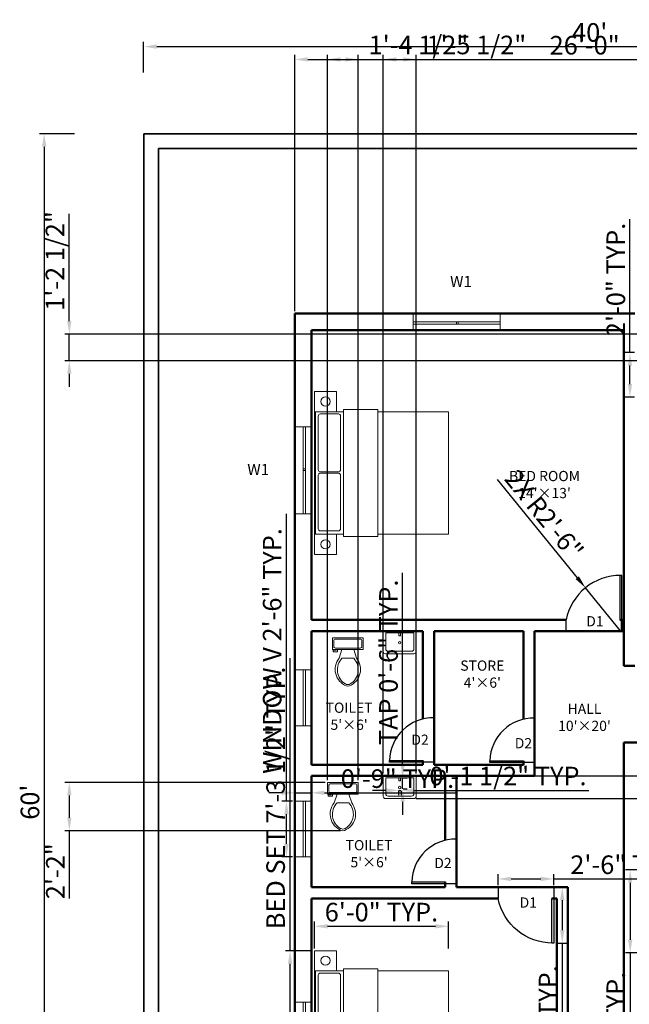
# Model space of a CAD drawing. Units: inches. Extents: x 452 to 1041, y 578 to 1412.
# Tile 2 of 3: x 452 to 780, y 881 to 1412. Entities that reach past the tile are written whole.
import ezdxf

# ---------------------------------------------------------------- set-up
doc = ezdxf.new("R2010")
doc.units = ezdxf.units.IN
doc.linetypes.add('ACAD_ISO03W100', pattern=[30, 12, -18])
doc.layers.get('Defpoints').update_dxf_attribs({"linetype": 'ACAD_ISO03W100'})
for name, color, linetype, lineweight in [('A-ANNO-DIMS', 2, 'Continuous', 18), ('A-ANNO-TEXT', 7, 'Continuous', 18), ('A-AREA-IDEN', 7, 'Continuous', 25), ('A-DOOR', 3, 'Continuous', 25), ('A-FLOR-FIXT', 9, 'Continuous', 18), ('A-FURN', 8, 'Continuous', 18), ('A-GLAZ', 160, 'Continuous', 20), ('A-WALL', 7, 'Continuous', 50), ('C-PROP', 7, 'Continuous', 35)]:
    doc.layers.add(name, color=color, linetype=linetype, lineweight=lineweight)
doc.styles.get("Standard").update_dxf_attribs({"font": 'times.ttf'})
doc.dimstyles.new('ISO-25', dxfattribs={"dimscale": 2, "dimtxt": 5, "dimasz": 3.5, "dimexe": 1.25, "dimexo": 0.625, "dimtad": 1, "dimdsep": 46, "dimlunit": 3, "dimtxsty": 'Standard', "dimcen": 2.5, "dimadec": 0, "dimazin": 0, "dimtfac": 1, "dimtmove": 0, "dimatfit": 3, "dimfxl": 1, "dimarcsym": 0})

# ---------------------------------------------------------------- blocks, each defined once
blk = doc.blocks.new('*U2')
for p, q in [((9.5, -6), (9.5, -2)), ((-10, -8.5), (-8, -8.5)), ((-10, -9.5), (-10, -8.5)), ((-7, -9.5), (-10, -9.5)), ((-8, -8.5), (-8, -8)), ((-7, -8), (-7, -9.5)), ((-4, -8), (-6, -14)), ((4, -8), (6, -14)), ((4, -14), (-4, -14))]:
    blk.add_line(p, q)
blk.add_lwpolyline([(10.5, -8), (10.5, 0), (-10.5, 0), (-10.5, -8)], close=True)
for points in [[(-9.5, -2), (-9.5, -6)], [(8.5, -1), (-8.5, -1)], [(-8.5, -7), (8.5, -7)]]:
    blk.add_lwpolyline(points)
for centre, radius, start, end in [((-8.62, -1.88), 0.884, 81.8699, 188.1301), ((-8.62, -6.12), 0.884, 171.8699, 278.1301), ((8.62, -1.88), 0.884, 351.8699, 98.1301), ((8.62, -6.12), 0.884, 261.8699, 8.1301), ((3.52, -21.58), 12.17, 141.46911, 247.97143), ((4.2, -21.82), 11.33, 136.36773, 238.94682), ((-3.52, -21.58), 12.17, 292.02843, 38.53071), ((-4.2, -21.82), 11.33, 301.05301, 43.63209), ((0, -27.88), 4, 245.73182, 294.26817), ((0, -29), 4, 254.86053, 285.13947)]:
    blk.add_arc(centre, radius, start, end)
blk = doc.blocks.new('D1')
for p, q in [((734.6, 1191.77), (733.6, 1191.77)), ((733.6, 1191.77), (733.6, 1167.77)), ((734.6, 1161.77), (734.6, 1191.77)), ((704.6, 1161.77), (704.6, 1167.77))]:
    blk.add_line(p, q)
blk.add_arc((733.85, 1161.94), 29.82, 89.5197, 168.7411)
blk = doc.blocks.new('W')
for p, q in [((913.24, 916.29), (913.24, 963.09)), ((913.24, 963.09), (922.24, 963.09)), ((917.74, 963.09), (917.74, 916.29)), ((918.94, 963.09), (918.94, 916.29)), ((922.24, 963.09), (922.24, 916.29)), ((917.74, 940.48), (918.94, 940.48)), ((917.74, 939.69), (918.94, 939.69)), ((922.24, 916.29), (913.24, 916.29))]:
    blk.add_line(p, q)
blk = doc.blocks.new('V')
for p, q in [((599.59, 961.66), (599.59, 991.66)), ((599.59, 991.66), (608.59, 991.66)), ((604.09, 961.66), (604.09, 991.66)), ((604.09, 991.66), (605.29, 991.66)), ((605.29, 991.66), (605.29, 961.66)), ((608.59, 991.66), (608.59, 961.66)), ((608.59, 961.66), (599.59, 961.66)), ((608.59, 961.66), (604.09, 961.66))]:
    blk.add_line(p, q)
blk = doc.blocks.new('*D7')
at = {"layer": 'A-ANNO-DIMS', "color": 0, "lineweight": -2, "transparency": 16777216}
for p, q in [((518.29, 1383.36), (518.29, 1399.73)), ((525.29, 1397.23), (991.29, 1397.23)), ((998.29, 1383.36), (998.29, 1399.73))]:
    blk.add_line(p, q, dxfattribs=at)
at = {"layer": 'A-ANNO-DIMS', "color": 0, "lineweight": 70, "transparency": 16777216}
for points in [[(525.29, 1398.4), (525.29, 1396.06), (518.29, 1397.23)], [(991.29, 1398.4), (991.29, 1396.06), (998.29, 1397.23)]]:
    blk.add_solid(points, dxfattribs=at)
at = {"layer": 'Defpoints', "color": 0, "lineweight": 70, "transparency": 16777216}
for p in [(998.29, 1397.23), (518.29, 1382.11), (998.29, 1382.11)]:
    blk.add_point(p, dxfattribs=at)
at = {"layer": 'A-ANNO-DIMS', "color": 0, "transparency": 16777216, "insert": (758.29, 1403.57), "char_height": 10, "attachment_point": 5}
blk.add_mtext("40'", dxfattribs=at)
blk = doc.blocks.new('*D8')
at = {"layer": 'A-ANNO-DIMS', "color": 0, "lineweight": -2, "transparency": 16777216}
for p, q in [((481.13, 1350.33), (462.24, 1350.33)), ((464.74, 1343.33), (464.74, 637.33)), ((481.13, 630.33), (462.24, 630.33))]:
    blk.add_line(p, q, dxfattribs=at)
at = {"layer": 'A-ANNO-DIMS', "color": 0, "lineweight": 70, "transparency": 16777216}
for points in [[(463.58, 1343.33), (465.91, 1343.33), (464.74, 1350.33)], [(463.58, 637.33), (465.91, 637.33), (464.74, 630.33)]]:
    blk.add_solid(points, dxfattribs=at)
at = {"layer": 'Defpoints', "color": 0, "lineweight": 70, "transparency": 16777216}
for p in [(482.38, 1350.33), (464.74, 630.33), (482.38, 630.33)]:
    blk.add_point(p, dxfattribs=at)
at = {"layer": 'A-ANNO-DIMS', "color": 0, "transparency": 16777216, "insert": (458.41, 990.33), "char_height": 10, "attachment_point": 5, "rotation": 90}
blk.add_mtext("60'", dxfattribs=at)
blk = doc.blocks.new('BED-FRAME-AND-SIDE-TABLES')
for p, q in [((0, 76.85), (15.53, 76.85)), ((0, 10.85), (0, 76.85)), ((0.5, 76.85), (0.5, 10.85)), ((33.97, 76.85), (72, 76.85)), ((72, 76.85), (72, 10.85)), ((15.53, 10.85), (0, 10.85)), ((72, 10.85), (33.97, 10.85))]:
    blk.add_line(p, q)
for points in [[(0, 76.85), (11.87, 76.85), (11.87, 87.71), (0, 87.71)], [(15.53, 78), (33.97, 78), (33.97, 9.68), (15.53, 9.68)], [(0, 0), (11.87, 0), (11.87, 10.85), (0, 10.85)]]:
    blk.add_lwpolyline(points, close=True)
for centre in [(5.89, 82.36), (5.89, 5.42)]:
    blk.add_circle(centre, 2.46)
blk = doc.blocks.new('DOOR-D2-24IN')
for p, q in [((0, 0), (0, 24)), ((0, 24), (1, 24)), ((1, 24), (1, 6)), ((1, 6), (0, 6)), ((0, 0), (24, 0))]:
    blk.add_line(p, q)
blk.add_arc((0.44, 0.44), 23.57, 358.9406, 88.6428)
blk = doc.blocks.new('BASIN-FITTINGS')
blk.add_lwpolyline([(0.26, 5.96), (1.05, 5.96), (1.05, 4.28), (0.26, 4.28)], close=True)
blk.add_circle((0.67, 0.67), 0.671)
blk.add_circle((0.67, 0.67), 0.671)
blk = doc.blocks.new('*D20')
at = {"layer": 'A-ANNO-DIMS', "color": 0, "lineweight": -2, "transparency": 16777216}
for p, q in [((595.09, 990.85), (595.09, 1145.58)), ((598.34, 990.85), (592.59, 990.85)), ((595.09, 967.85), (595.09, 983.85)), ((598.34, 960.85), (592.59, 960.85))]:
    blk.add_line(p, q, dxfattribs=at)
at = {"layer": 'A-ANNO-DIMS', "color": 0, "lineweight": 70, "transparency": 16777216}
for points in [[(593.93, 983.85), (596.26, 983.85), (595.09, 990.85)], [(593.93, 967.85), (596.26, 967.85), (595.09, 960.85)]]:
    blk.add_solid(points, dxfattribs=at)
at = {"layer": 'Defpoints', "color": 0, "lineweight": 70, "transparency": 16777216}
for p in [(595.09, 990.85), (599.59, 990.85), (599.59, 960.85)]:
    blk.add_point(p, dxfattribs=at)
at = {"layer": 'A-ANNO-DIMS', "color": 0, "transparency": 16777216, "insert": (588.73, 1071.72), "char_height": 10, "attachment_point": 5, "rotation": 90}
blk.add_mtext('WINDOW V 2\'-6" TYP.', dxfattribs=at)
blk = doc.blocks.new('*D21')
at = {"layer": 'A-ANNO-DIMS', "color": 0, "lineweight": -2, "transparency": 16777216}
for p, q in [((599.59, 992.1), (599.59, 997.85)), ((608.59, 992.1), (608.59, 997.85)), ((592.59, 995.35), (585.59, 995.35)), ((599.59, 995.35), (608.59, 995.35)), ((615.59, 995.35), (687.16, 995.35))]:
    blk.add_line(p, q, dxfattribs=at)
at = {"layer": 'A-ANNO-DIMS', "color": 0, "lineweight": 70, "transparency": 16777216}
for points in [[(592.59, 996.52), (592.59, 994.18), (599.59, 995.35)], [(615.59, 996.52), (615.59, 994.18), (608.59, 995.35)]]:
    blk.add_solid(points, dxfattribs=at)
at = {"layer": 'Defpoints', "color": 0, "lineweight": 70, "transparency": 16777216}
for p in [(608.59, 995.35), (599.59, 990.85), (608.59, 990.85)]:
    blk.add_point(p, dxfattribs=at)
at = {"layer": 'A-ANNO-DIMS', "color": 0, "transparency": 16777216, "insert": (654.88, 1001.7), "char_height": 10, "attachment_point": 5}
blk.add_mtext('0\'-9" TYP.', dxfattribs=at)
blk = doc.blocks.new('*D22')
at = {"layer": 'A-ANNO-DIMS', "color": 0, "lineweight": -2, "transparency": 16777216}
for p, q in [((740.23, 944.45), (746, 944.45)), ((743.5, 937.45), (743.5, 921.33)), ((740.23, 914.33), (746, 914.33)), ((743.5, 914.33), (743.5, 775.21))]:
    blk.add_line(p, q, dxfattribs=at)
at = {"layer": 'A-ANNO-DIMS', "color": 0, "lineweight": 70, "transparency": 16777216}
for points in [[(742.34, 937.45), (744.67, 937.45), (743.5, 944.45)], [(742.34, 921.33), (744.67, 921.33), (743.5, 914.33)]]:
    blk.add_solid(points, dxfattribs=at)
at = {"layer": 'Defpoints', "color": 0, "lineweight": 70, "transparency": 16777216}
for p in [(738.98, 944.45), (738.98, 914.33), (743.5, 914.33)]:
    blk.add_point(p, dxfattribs=at)
at = {"layer": 'A-ANNO-DIMS', "color": 0, "transparency": 16777216, "insert": (737.14, 841.27), "char_height": 10, "attachment_point": 5, "rotation": 90}
blk.add_mtext('DOOR D1 2\'-6" TYP.', dxfattribs=at)
blk = doc.blocks.new('*D23')
at = {"layer": 'A-ANNO-DIMS', "color": 0, "lineweight": -2, "transparency": 16777216}
for p, q in [((708.98, 945.7), (708.98, 951.47)), ((738.98, 945.7), (738.98, 951.47)), ((715.98, 948.97), (731.98, 948.97)), ((738.98, 948.97), (810.77, 948.97))]:
    blk.add_line(p, q, dxfattribs=at)
at = {"layer": 'A-ANNO-DIMS', "color": 0, "lineweight": 70, "transparency": 16777216}
for points in [[(715.98, 950.14), (715.98, 947.8), (708.98, 948.97)], [(731.98, 950.14), (731.98, 947.8), (738.98, 948.97)]]:
    blk.add_solid(points, dxfattribs=at)
at = {"layer": 'Defpoints', "color": 0, "lineweight": 70, "transparency": 16777216}
for p in [(708.98, 944.45), (738.98, 948.97), (738.98, 944.45)]:
    blk.add_point(p, dxfattribs=at)
at = {"layer": 'A-ANNO-DIMS', "color": 0, "transparency": 16777216, "insert": (778.38, 955.32), "char_height": 10, "attachment_point": 5}
blk.add_mtext('2\'-6" TYP.', dxfattribs=at)
blk = doc.blocks.new('*D25')
at = {"layer": 'A-ANNO-DIMS', "color": 0, "lineweight": -2, "transparency": 16777216}
for p, q in [((779.96, 1232.45), (779.96, 1304.24)), ((782.34, 1232.45), (777.46, 1232.45)), ((779.96, 1215.45), (779.96, 1225.45)), ((782.34, 1208.45), (777.46, 1208.45))]:
    blk.add_line(p, q, dxfattribs=at)
at = {"layer": 'A-ANNO-DIMS', "color": 0, "lineweight": 70, "transparency": 16777216}
for points in [[(778.79, 1225.45), (781.12, 1225.45), (779.96, 1232.45)], [(778.79, 1215.45), (781.12, 1215.45), (779.96, 1208.45)]]:
    blk.add_solid(points, dxfattribs=at)
at = {"layer": 'Defpoints', "color": 0, "lineweight": 70, "transparency": 16777216}
for p in [(779.96, 1232.45), (783.59, 1232.45), (783.59, 1208.45)]:
    blk.add_point(p, dxfattribs=at)
at = {"layer": 'A-ANNO-DIMS', "color": 0, "transparency": 16777216, "insert": (773.61, 1271.84), "char_height": 10, "attachment_point": 5, "rotation": 90}
blk.add_mtext('2\'-0" TYP.', dxfattribs=at)
blk = doc.blocks.new('*D30')
at = {"layer": 'A-ANNO-DIMS', "color": 0, "lineweight": -2, "transparency": 16777216}
for p, q in [((657.65, 1010.49), (657.65, 1113.74)), ((657.65, 997.53), (657.65, 1003.49)), ((658.01, 1003.49), (660.15, 1003.49)), ((658.01, 997.53), (660.15, 997.53)), ((657.65, 990.53), (657.65, 983.53))]:
    blk.add_line(p, q, dxfattribs=at)
at = {"layer": 'A-ANNO-DIMS', "color": 0, "lineweight": 70, "transparency": 16777216}
for points in [[(656.48, 1010.49), (658.82, 1010.49), (657.65, 1003.49)], [(656.48, 990.53), (658.82, 990.53), (657.65, 997.53)]]:
    blk.add_solid(points, dxfattribs=at)
at = {"layer": 'Defpoints', "color": 0, "lineweight": 70, "transparency": 16777216}
for p in [(656.76, 1003.49), (657.65, 1003.49), (656.76, 997.53)]:
    blk.add_point(p, dxfattribs=at)
at = {"layer": 'A-ANNO-DIMS', "color": 0, "transparency": 16777216, "insert": (651.3, 1065.62), "char_height": 10, "attachment_point": 5, "rotation": 90}
blk.add_mtext('TAP 0\'-6" TYP.', dxfattribs=at)
blk = doc.blocks.new('*D31')
at = {"layer": 'A-ANNO-DIMS', "color": 0, "lineweight": -2, "transparency": 16777216}
for p, q in [((648.41, 996.64), (641.41, 996.64)), ((655.41, 996.64), (656.76, 996.64)), ((655.41, 996.28), (655.41, 994.14)), ((656.76, 996.28), (656.76, 994.14)), ((663.76, 996.64), (757.89, 996.64))]:
    blk.add_line(p, q, dxfattribs=at)
at = {"layer": 'A-ANNO-DIMS', "color": 0, "lineweight": 70, "transparency": 16777216}
for points in [[(648.41, 997.8), (648.41, 995.47), (655.41, 996.64)], [(663.76, 997.8), (663.76, 995.47), (656.76, 996.64)]]:
    blk.add_solid(points, dxfattribs=at)
at = {"layer": 'Defpoints', "color": 0, "lineweight": 70, "transparency": 16777216}
for p in [(655.41, 997.53), (656.76, 997.53), (656.76, 996.64)]:
    blk.add_point(p, dxfattribs=at)
at = {"layer": 'A-ANNO-DIMS', "color": 0, "transparency": 16777216, "insert": (714.32, 1003.11), "char_height": 10, "attachment_point": 5}
blk.add_mtext('0\'-1 1/2" TYP.', dxfattribs=at)
blk = doc.blocks.new('*D32')
at = {"layer": 'A-ANNO-DIMS', "color": 0, "lineweight": -2, "transparency": 16777216}
for p, q in [((785.53, 953.88), (777.57, 953.88)), ((780.07, 946.88), (780.07, 916.19)), ((785.53, 909.19), (777.57, 909.19)), ((780.07, 909.19), (780.07, 774.01))]:
    blk.add_line(p, q, dxfattribs=at)
at = {"layer": 'A-ANNO-DIMS', "color": 0, "lineweight": 70, "transparency": 16777216}
for points in [[(778.91, 946.88), (781.24, 946.88), (780.07, 953.88)], [(778.91, 916.19), (781.24, 916.19), (780.07, 909.19)]]:
    blk.add_solid(points, dxfattribs=at)
at = {"layer": 'Defpoints', "color": 0, "lineweight": 70, "transparency": 16777216}
for p in [(786.78, 953.88), (780.07, 909.19), (786.78, 909.19)]:
    blk.add_point(p, dxfattribs=at)
at = {"layer": 'A-ANNO-DIMS', "color": 0, "transparency": 16777216, "insert": (773.59, 838.1), "char_height": 10, "attachment_point": 5, "rotation": 90}
blk.add_mtext('SOFA 3\'-8 1/2" TYP.', dxfattribs=at)
blk = doc.blocks.new('*D34')
at = {"layer": 'A-ANNO-DIMS', "color": 0, "lineweight": -2, "transparency": 16777216}
for p, q in [((597.08, 910.3), (597.08, 1067.89)), ((608.99, 910.3), (594.58, 910.3)), ((597.08, 829.6), (597.08, 903.3)), ((608.99, 822.6), (594.58, 822.6))]:
    blk.add_line(p, q, dxfattribs=at)
at = {"layer": 'A-ANNO-DIMS', "color": 0, "lineweight": 70, "transparency": 16777216}
for points in [[(595.92, 903.3), (598.25, 903.3), (597.08, 910.3)], [(595.92, 829.6), (598.25, 829.6), (597.08, 822.6)]]:
    blk.add_solid(points, dxfattribs=at)
at = {"layer": 'Defpoints', "color": 0, "lineweight": 70, "transparency": 16777216}
for p in [(597.08, 910.3), (610.24, 910.3), (610.24, 822.6)]:
    blk.add_point(p, dxfattribs=at)
at = {"layer": 'A-ANNO-DIMS', "color": 0, "transparency": 16777216, "insert": (590.59, 992.6), "char_height": 10, "attachment_point": 5, "rotation": 90}
blk.add_mtext('BED SET 7\'-3 1/2" TYP.', dxfattribs=at)
blk = doc.blocks.new('*D35')
at = {"layer": 'A-ANNO-DIMS', "color": 0, "lineweight": -2, "transparency": 16777216}
for p, q in [((610.24, 911.55), (610.24, 925.96)), ((617.24, 923.46), (675.24, 923.46)), ((682.24, 911.55), (682.24, 925.96))]:
    blk.add_line(p, q, dxfattribs=at)
at = {"layer": 'A-ANNO-DIMS', "color": 0, "lineweight": 70, "transparency": 16777216}
for points in [[(617.24, 924.63), (617.24, 922.29), (610.24, 923.46)], [(675.24, 924.63), (675.24, 922.29), (682.24, 923.46)]]:
    blk.add_solid(points, dxfattribs=at)
at = {"layer": 'Defpoints', "color": 0, "lineweight": 70, "transparency": 16777216}
for p in [(682.24, 923.46), (610.24, 910.3), (682.24, 910.3)]:
    blk.add_point(p, dxfattribs=at)
at = {"layer": 'A-ANNO-DIMS', "color": 0, "transparency": 16777216, "insert": (646.24, 929.81), "char_height": 10, "attachment_point": 5}
blk.add_mtext('6\'-0" TYP.', dxfattribs=at)
blk = doc.blocks.new('*D38')
at = {"layer": 'A-ANNO-DIMS', "color": 0, "lineweight": -2, "transparency": 16777216}
for p, q in [((599.59, 1254.7), (599.59, 1392.83)), ((606.59, 1390.33), (904.59, 1390.33)), ((911.59, 1254.7), (911.59, 1392.83))]:
    blk.add_line(p, q, dxfattribs=at)
at = {"layer": 'A-ANNO-DIMS', "color": 0, "lineweight": 70, "transparency": 16777216}
for points in [[(606.59, 1391.5), (606.59, 1389.17), (599.59, 1390.33)], [(904.59, 1391.5), (904.59, 1389.17), (911.59, 1390.33)]]:
    blk.add_solid(points, dxfattribs=at)
at = {"layer": 'Defpoints', "color": 0, "lineweight": 70, "transparency": 16777216}
for p in [(911.59, 1390.33), (599.59, 1253.45), (911.59, 1253.45)]:
    blk.add_point(p, dxfattribs=at)
at = {"layer": 'A-ANNO-DIMS', "color": 0, "transparency": 16777216, "insert": (755.59, 1396.67), "char_height": 10, "attachment_point": 5}
blk.add_mtext('26\'-0"', dxfattribs=at)
blk = doc.blocks.new('*D51')
at = {"layer": 'A-ANNO-DIMS', "color": 0, "lineweight": -2, "transparency": 16777216}
for p, q in [((478.29, 1249.43), (478.29, 1307.15)), ((845.22, 1242.43), (475.79, 1242.43)), ((478.29, 1228), (478.29, 1242.43)), ((845.22, 1228), (475.79, 1228)), ((478.29, 1221), (478.29, 1214))]:
    blk.add_line(p, q, dxfattribs=at)
at = {"layer": 'A-ANNO-DIMS', "color": 0, "lineweight": 70, "transparency": 16777216}
for points in [[(477.13, 1249.43), (479.46, 1249.43), (478.29, 1242.43)], [(477.13, 1221), (479.46, 1221), (478.29, 1228)]]:
    blk.add_solid(points, dxfattribs=at)
at = {"layer": 'Defpoints', "color": 0, "lineweight": 70, "transparency": 16777216}
for p in [(478.29, 1242.43), (846.47, 1242.43), (846.47, 1228)]:
    blk.add_point(p, dxfattribs=at)
at = {"layer": 'A-ANNO-DIMS', "color": 0, "transparency": 16777216, "insert": (471.82, 1281.79), "char_height": 10, "attachment_point": 5, "rotation": 90}
blk.add_mtext('1\'-2 1/2"', dxfattribs=at)
blk = doc.blocks.new('*D54')
at = {"layer": 'A-ANNO-DIMS', "color": 0, "lineweight": -2, "transparency": 16777216}
for p, q in [((617.2, 1002.23), (617.2, 1392.83)), ((624.2, 1390.33), (626.78, 1390.33)), ((633.78, 1002.23), (633.78, 1392.83)), ((633.78, 1390.33), (691.5, 1390.33))]:
    blk.add_line(p, q, dxfattribs=at)
at = {"layer": 'A-ANNO-DIMS', "color": 0, "lineweight": 70, "transparency": 16777216}
for points in [[(624.2, 1391.5), (624.2, 1389.17), (617.2, 1390.33)], [(626.78, 1391.5), (626.78, 1389.17), (633.78, 1390.33)]]:
    blk.add_solid(points, dxfattribs=at)
at = {"layer": 'Defpoints', "color": 0, "lineweight": 70, "transparency": 16777216}
for p in [(633.78, 1390.33), (617.2, 1000.98), (633.78, 1000.98)]:
    blk.add_point(p, dxfattribs=at)
at = {"layer": 'A-ANNO-DIMS', "color": 0, "transparency": 16777216, "insert": (666.14, 1396.81), "char_height": 10, "attachment_point": 5}
blk.add_mtext('1\'-4 1/2"', dxfattribs=at)
blk = doc.blocks.new('*D55')
at = {"layer": 'A-ANNO-DIMS', "color": 0, "lineweight": -2, "transparency": 16777216}
for p, q in [((615.95, 1000.98), (475.79, 1000.98)), ((478.29, 993.98), (478.29, 981.92)), ((624.24, 974.92), (475.79, 974.92)), ((478.29, 974.92), (478.29, 938.35))]:
    blk.add_line(p, q, dxfattribs=at)
at = {"layer": 'A-ANNO-DIMS', "color": 0, "lineweight": 70, "transparency": 16777216}
for points in [[(477.13, 993.98), (479.46, 993.98), (478.29, 1000.98)], [(477.13, 981.92), (479.46, 981.92), (478.29, 974.92)]]:
    blk.add_solid(points, dxfattribs=at)
at = {"layer": 'Defpoints', "color": 0, "lineweight": 70, "transparency": 16777216}
for p in [(617.2, 1000.98), (478.29, 974.92), (625.49, 974.92)]:
    blk.add_point(p, dxfattribs=at)
at = {"layer": 'A-ANNO-DIMS', "color": 0, "transparency": 16777216, "insert": (472.04, 953.14), "char_height": 10, "attachment_point": 5, "rotation": 90}
blk.add_mtext('2\'-2"', dxfattribs=at)
blk = doc.blocks.new('*D56')
at = {"layer": 'A-ANNO-DIMS', "color": 0, "lineweight": -2, "transparency": 16777216}
for p, q in [((647.22, 1005.7), (647.22, 1392.83)), ((654.22, 1390.33), (657.93, 1390.33)), ((664.93, 1005.7), (664.93, 1392.83)), ((664.93, 1390.33), (722.65, 1390.33))]:
    blk.add_line(p, q, dxfattribs=at)
at = {"layer": 'A-ANNO-DIMS', "color": 0, "lineweight": 70, "transparency": 16777216}
for points in [[(654.22, 1391.5), (654.22, 1389.17), (647.22, 1390.33)], [(657.93, 1391.5), (657.93, 1389.17), (664.93, 1390.33)]]:
    blk.add_solid(points, dxfattribs=at)
at = {"layer": 'Defpoints', "color": 0, "lineweight": 70, "transparency": 16777216}
for p in [(664.93, 1390.33), (647.22, 1004.45), (664.93, 1004.45)]:
    blk.add_point(p, dxfattribs=at)
at = {"layer": 'A-ANNO-DIMS', "color": 0, "transparency": 16777216, "insert": (697.29, 1396.81), "char_height": 10, "attachment_point": 5}
blk.add_mtext('1\'-5 1/2"', dxfattribs=at)
blk = doc.blocks.new('*D57')
at = {"layer": 'A-ANNO-DIMS', "color": 0, "lineweight": -2, "transparency": 16777216}
for p, q in [((1038.29, 1011.45), (1038.29, 1018.45)), ((666.18, 1004.45), (1040.79, 1004.45)), ((1038.29, 1004.45), (1038.29, 992.25)), ((664.98, 992.25), (1040.79, 992.25)), ((1038.29, 985.25), (1038.29, 950.09))]:
    blk.add_line(p, q, dxfattribs=at)
at = {"layer": 'A-ANNO-DIMS', "color": 0, "lineweight": 70, "transparency": 16777216}
for points in [[(1037.13, 1011.45), (1039.46, 1011.45), (1038.29, 1004.45)], [(1037.13, 985.25), (1039.46, 985.25), (1038.29, 992.25)]]:
    blk.add_solid(points, dxfattribs=at)
at = {"layer": 'Defpoints', "color": 0, "lineweight": 70, "transparency": 16777216}
for p in [(664.93, 1004.45), (663.73, 992.25), (1038.29, 992.25)]:
    blk.add_point(p, dxfattribs=at)
at = {"layer": 'A-ANNO-DIMS', "color": 0, "transparency": 16777216, "insert": (1031.96, 964.17), "char_height": 10, "attachment_point": 5, "rotation": 90}
blk.add_mtext('1\'-0"', dxfattribs=at)
blk = doc.blocks.new('*D58')
at = {"layer": 'A-ANNO-DIMS', "color": 0, "lineweight": -2, "transparency": 16777216}
for p, q in [((708.59, 1164.06), (751.6, 1111.19)), ((774.84, 1082.63), (756.02, 1105.76))]:
    blk.add_line(p, q, dxfattribs=at)
at = {"layer": 'A-ANNO-DIMS', "color": 0, "lineweight": 70, "transparency": 16777216}
blk.add_solid([(752.51, 1111.93), (750.7, 1110.46), (756.02, 1105.76)], dxfattribs=at)
at = {"layer": 'Defpoints', "color": 0, "lineweight": 70, "transparency": 16777216}
for p in [(756.02, 1105.76), (774.84, 1082.63)]:
    blk.add_point(p, dxfattribs=at)
at = {"layer": 'A-ANNO-DIMS', "color": 0, "transparency": 16777216, "insert": (732.8, 1144.34), "char_height": 10, "attachment_point": 5, "rotation": 309.1309}
blk.add_mtext('2X R2\'-6"', dxfattribs=at)

msp = doc.modelspace()

# ---------------------------------------------------------------- linework, layer by layer
at = {"layer": 'A-DOOR'}
for p, q in [((775.593, 1112.451), (774.593, 1112.451)), ((774.593, 1112.451), (774.593, 1088.451)), ((775.593, 1082.451), (775.593, 1112.451)), ((745.593, 1082.451), (745.593, 1088.451)), ((775.593, 1082.451), (745.593, 1082.451))]:
    msp.add_line(p, q, dxfattribs=at)
msp.add_arc((774.843, 1082.628), 29.824, 89.51971, 168.74109, dxfattribs=at)
at = {"layer": 'A-FLOR-FIXT'}
for points in [[(647.216, 1082.451), (664.929, 1082.451), (664.929, 1071.451, -0.4142136), (663.729, 1070.251), (648.416, 1070.251, -0.4142136), (647.216, 1071.451)], [(648.586, 1081.495), (663.681, 1081.495), (663.681, 1072.828, -0.4142136), (662.481, 1071.628), (649.786, 1071.628, -0.4142136), (648.586, 1072.828)], [(647.216, 1004.451), (664.929, 1004.451), (664.929, 993.451, -0.4142136), (663.729, 992.251), (648.416, 992.251, -0.4142136), (647.216, 993.451)], [(648.586, 1003.495), (663.681, 1003.495), (663.681, 994.828, -0.4142136), (662.481, 993.628), (649.786, 993.628, -0.4142136), (648.586, 994.828)]]:
    msp.add_lwpolyline(points, format="xyb", close=True, dxfattribs=at)
at = {"layer": 'A-FURN'}
for points in [[(613.446, 1168.239), (623.072, 1168.239, 0.4142136), (624.272, 1169.439), (624.272, 1198.216, 0.4142136), (623.072, 1199.416), (613.446, 1199.416, 0.4142136), (612.246, 1198.216), (612.246, 1169.439, 0.4142136)], [(613.446, 1136.403), (623.072, 1136.403, 0.4142136), (624.272, 1137.603), (624.272, 1166.38, 0.4142136), (623.072, 1167.58), (613.446, 1167.58, 0.4142136), (612.246, 1166.38), (612.246, 1137.603, 0.4142136)], [(613.452, 867.109), (623.078, 867.109, 0.4142136), (624.278, 868.309), (624.278, 897.087, 0.4142136), (623.078, 898.287), (613.452, 898.287, 0.4142136), (612.252, 897.087), (612.252, 868.309, 0.4142136)]]:
    msp.add_lwpolyline(points, format="xyb", close=True, dxfattribs=at)
at = {"layer": 'A-WALL'}
for p, q in [((599.593, 1253.451), (599.593, 1082.451)), ((599.593, 1253.451), (776.593, 1253.451)), ((776.593, 1253.451), (782.593, 1253.451)), ((608.593, 1244.451), (776.593, 1244.451)), ((608.593, 1244.451), (608.593, 1088.451)), ((776.593, 1244.451), (776.593, 1088.451)), ((745.593, 1088.451), (608.593, 1088.451)), ((776.593, 1088.451), (774.593, 1088.451)), ((775.593, 1082.451), (775.593, 1088.451)), ((776.593, 1063.736), (776.593, 1088.451)), ((599.593, 1082.451), (599.593, 1004.451)), ((668.593, 1082.451), (608.593, 1082.451)), ((608.593, 1082.451), (608.593, 1010.451)), ((668.593, 1082.451), (608.593, 1082.451)), ((668.593, 1035.12), (668.593, 1082.451)), ((674.593, 1010.451), (674.593, 1082.451)), ((674.593, 1082.451), (722.593, 1082.451)), ((722.593, 1082.451), (674.593, 1082.451)), ((722.593, 1082.451), (722.593, 1034.977)), ((728.593, 1004.451), (728.593, 1082.451)), ((776.593, 1082.451), (728.593, 1082.451)), ((776.593, 1082.451), (775.593, 1082.451)), ((776.593, 1063.736), (782.593, 1063.736)), ((902.593, 1022.451), (776.593, 1022.451)), ((776.593, 1013.451), (776.593, 1022.451)), ((776.593, 847.904), (776.593, 1013.451)), ((608.593, 1010.451), (668.593, 1010.451)), ((668.593, 1010.451), (668.593, 1012.773)), ((722.593, 1010.451), (674.593, 1010.451)), ((722.593, 1012.63), (722.593, 1010.451)), ((599.593, 1004.451), (599.593, 944.451)), ((608.593, 1004.451), (674.593, 1004.451)), ((608.593, 1004.451), (608.593, 944.451)), ((674.593, 1004.451), (722.593, 1004.451)), ((680.593, 969.751), (680.593, 1004.451)), ((686.593, 944.451), (686.593, 1004.451)), ((722.593, 1004.451), (728.593, 1004.451)), ((599.593, 944.451), (599.593, 938.451)), ((608.593, 944.451), (680.593, 944.451)), ((680.593, 944.451), (680.593, 947.405)), ((686.593, 944.451), (740.593, 944.451)), ((740.593, 944.451), (746.593, 944.451)), ((746.593, 944.451), (746.593, 794.451)), ((599.593, 785.451), (599.593, 938.451)), ((608.593, 938.451), (686.593, 938.451)), ((608.593, 938.451), (608.593, 794.451)), ((708.984, 938.451), (686.593, 938.451)), ((740.593, 938.451), (737.984, 938.451)), ((740.593, 794.451), (740.593, 938.451))]:
    msp.add_line(p, q, dxfattribs=at)
at = {"layer": 'C-PROP'}
for p, q in [((518.294, 1350.334), (998.294, 1350.334)), ((518.294, 630.334), (518.294, 1350.334)), ((526.294, 1342.334), (990.294, 1342.334)), ((526.294, 638.334), (526.294, 1342.334))]:
    msp.add_line(p, q, dxfattribs=at)

# ---------------------------------------------------------------- block references
at = {"layer": 'A-DOOR'}
for p, rotation in [((674.593, 1011.773), 90.00000000000038), ((728.593, 1011.63), 90.00000000000026), ((686.593, 946.404), 90.00000000000038)]:
    msp.add_blockref('DOOR-D2-24IN', p, dxfattribs=dict(at, rotation=rotation))
at = {"layer": 'A-DOOR', "xscale": -1, "rotation": 180}
msp.add_blockref('D1', (4.385, 2106.218), dxfattribs=at)
at = {"layer": 'A-FLOR-FIXT', "xscale": 0.7895724227718148, "yscale": 0.7895724227718148, "zscale": 0.7895724227718148}
for p in [(628.155, 1078.855), (625.491, 1000.978)]:
    msp.add_blockref('*U2', p, dxfattribs=at)
at = {"layer": 'A-FLOR-FIXT'}
for p in [(655.415, 1075.53), (655.415, 997.53)]:
    msp.add_blockref('BASIN-FITTINGS', p, dxfattribs=at)
at = {"layer": 'A-FURN'}
for p in [(610.232, 1123.727), (610.239, 822.597)]:
    msp.add_blockref('BED-FRAME-AND-SIDE-TABLES', p, dxfattribs=at)
at = {"layer": 'A-GLAZ', "rotation": 270}
msp.add_blockref('W', (-253.051, 2166.694), dxfattribs=at)
at = {"layer": 'A-GLAZ'}
for name, p in [('W', (-313.65, 229.309)), ('V', (0, 69.846)), ('V', (0, -0.815)), ('W', (-313.65, -80.554))]:
    msp.add_blockref(name, p, dxfattribs=at)

# ---------------------------------------------------------------- texts
at = {"layer": 'A-ANNO-TEXT', "attachment_point": 1}
for s, insert, char_height in [('W1', (683.173, 1273.753), 6), ('W1', (574.06, 1172.457), 6), ('D1', (756.426, 1090.499), 5.5), ('D2', (662.345, 1026.699), 5.5), ('D2', (717.972, 1024.833), 5.5), ('D2', (674.665, 960.288), 5.5), ('D1', (720.586, 939.021), 5.5)]:
    msp.add_mtext_dynamic_manual_height_columns(s, width=337.44086, gutter_width=12.5, heights=[0], dxfattribs=dict(at, insert=insert, char_height=char_height))
at = {"layer": 'A-AREA-IDEN', "char_height": 5.5, "attachment_point": 1}
for s, insert in [("\\pxqc;BED ROOM \\P14'×13'", (565.256, 1168.708)), ("\\pxqc;STORE\\P4'×6'", (531.801, 1066.618)), ("\\pxqc;TOILET\\P5'×6'", (460.112, 1043.931)), ("\\pxqc;HALL \\P10'×20'", (586.763, 1043.334)), ("\\pxqc;TOILET\\P5'×6'", (470.865, 969.901))]:
    msp.add_mtext_dynamic_manual_height_columns(s, width=337.44086, gutter_width=12.5, heights=[0], dxfattribs=dict(at, insert=insert))

# ---------------------------------------------------------------- dimensions: what is measured, and where the dimension line sits
at = {"layer": 'A-ANNO-DIMS'}
for base, p1, p2, override, picture, middle in [((633.781, 1390.334), (617.2, 1000.978), (633.781, 1000.978), {"dimdec": 1, "dimlfac": 1, "dimrnd": 0, "dimzin": 1, "dimdsep": 46, "dimlunit": 4, "dimfrac": 2}, '*D54', (666.141, 1396.811)), ((664.929, 1390.334), (647.216, 1004.451), (664.929, 1004.451), {"dimdec": 1, "dimlfac": 1, "dimrnd": 0, "dimzin": 1, "dimdsep": 46, "dimlunit": 4, "dimfrac": 2}, '*D56', (697.289, 1396.811)), ((998.294, 1397.23), (518.294, 1382.109), (998.294, 1382.109), {"dimclrd": 0, "dimclre": 0, "dimclrt": 0}, '*D7', (758.294, 1403.567)), ((911.593, 1390.334), (599.593, 1253.451), (911.593, 1253.451), {"dimdec": 1, "dimlfac": 1, "dimrnd": 0, "dimzin": 1, "dimdsep": 46, "dimlunit": 4, "dimfrac": 2}, '*D38', (755.593, 1396.671))]:
    dim = msp.add_linear_dim(base=base, p1=p1, p2=p2, dimstyle='ISO-25', override=override, dxfattribs=at)
    dim.commit()
    dim.dimension.update_dxf_attribs({"geometry": picture, "text_midpoint": middle})
for base, p1, p2, override, picture, middle in [((464.745, 630.334), (482.382, 1350.334), (482.382, 630.334), {"dimclrd": 0, "dimclre": 0, "dimclrt": 0}, '*D8', (458.408, 990.334)), ((478.294, 1242.43), (846.468, 1228.003), (846.468, 1242.43), {"dimdec": 1, "dimlfac": 1, "dimrnd": 0, "dimzin": 1, "dimdsep": 46, "dimlunit": 4, "dimfrac": 2}, '*D51', (471.817, 1281.79)), ((1038.294, 992.251), (664.929, 1004.451), (663.729, 992.251), {"dimdec": 1, "dimlfac": 1, "dimrnd": 0, "dimzin": 1, "dimdsep": 46, "dimlunit": 4, "dimfrac": 2}, '*D57', (1031.958, 964.171)), ((478.294, 974.922), (617.2, 1000.978), (625.491, 974.922), {"dimdec": 1, "dimlfac": 1, "dimrnd": 0, "dimzin": 1, "dimdsep": 46, "dimlunit": 4, "dimfrac": 2}, '*D55', (472.044, 953.136))]:
    dim = msp.add_linear_dim(base=base, p1=p1, p2=p2, angle=90, dimstyle='ISO-25', override=override, dxfattribs=at)
    dim.commit()
    dim.dimension.update_dxf_attribs({"geometry": picture, "text_midpoint": middle})
for base, p1, p2, angle, text, picture, middle in [((779.956, 1232.451), (783.593, 1208.451), (783.593, 1232.451), 90, '<> TYP.', '*D25', (773.605, 1271.843)), ((595.093, 990.848), (599.593, 960.848), (599.593, 990.848), 90, 'WINDOW V <> TYP.', '*D20', (588.732, 1071.716)), ((657.651, 1003.495), (656.757, 997.53), (656.757, 1003.495), 90, 'TAP <> TYP.', '*D30', (651.3, 1065.616)), ((597.082, 910.304), (610.239, 822.597), (610.239, 910.304), 90, 'BED SET <> TYP.', '*D34', (590.594, 992.595)), ((780.074, 909.191), (786.777, 953.88), (786.777, 909.191), 270, 'SOFA <> TYP.', '*D32', (773.586, 838.101)), ((743.502, 914.331), (738.984, 944.451), (738.984, 914.331), 270, 'DOOR D1 <> TYP.', '*D22', (737.14, 841.272))]:
    dim = msp.add_linear_dim(base=base, p1=p1, p2=p2, angle=angle, text=text, dimstyle='ISO-25', override={"dimdec": 1, "dimlfac": 1, "dimrnd": 0, "dimzin": 1, "dimdsep": 46, "dimlunit": 4, "dimfrac": 2}, dxfattribs=at)
    dim.commit()
    dim.dimension.update_dxf_attribs({"geometry": picture, "text_midpoint": middle})
dim = msp.add_radius_dim(center=(774.843, 1082.628), mpoint=(756.022, 1105.762), text='2X <>', dimstyle='ISO-25', override={"dimdec": 1, "dimlfac": 1, "dimrnd": 0, "dimzin": 1, "dimdsep": 46, "dimlunit": 4, "dimfrac": 2}, dxfattribs=at)
dim.commit()
dim.dimension.update_dxf_attribs({"geometry": '*D58', "text_midpoint": (732.803, 1144.342)})
for base, p1, p2, picture, middle in [((656.757, 996.636), (655.415, 997.53), (656.757, 997.53), '*D31', (714.321, 1003.113)), ((608.593, 995.348), (599.593, 990.848), (608.593, 990.848), '*D21', (654.878, 1001.699)), ((738.984, 948.969), (708.984, 944.451), (738.984, 944.451), '*D23', (778.376, 955.32)), ((682.239, 923.46), (610.239, 910.304), (682.239, 910.304), '*D35', (646.239, 929.811))]:
    dim = msp.add_linear_dim(base=base, p1=p1, p2=p2, text='<> TYP.', dimstyle='ISO-25', override={"dimdec": 1, "dimlfac": 1, "dimrnd": 0, "dimzin": 1, "dimdsep": 46, "dimlunit": 4, "dimfrac": 2}, dxfattribs=at)
    dim.commit()
    dim.dimension.update_dxf_attribs({"geometry": picture, "text_midpoint": middle})

doc.saveas('drawing.dxf')
